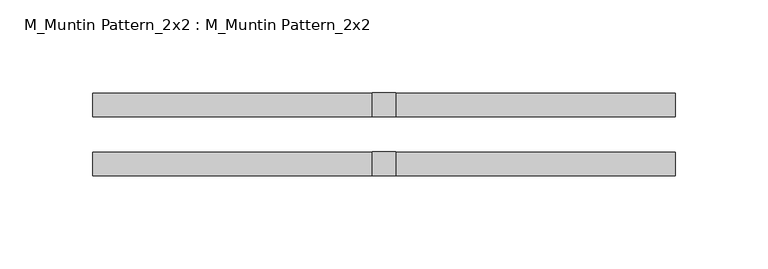
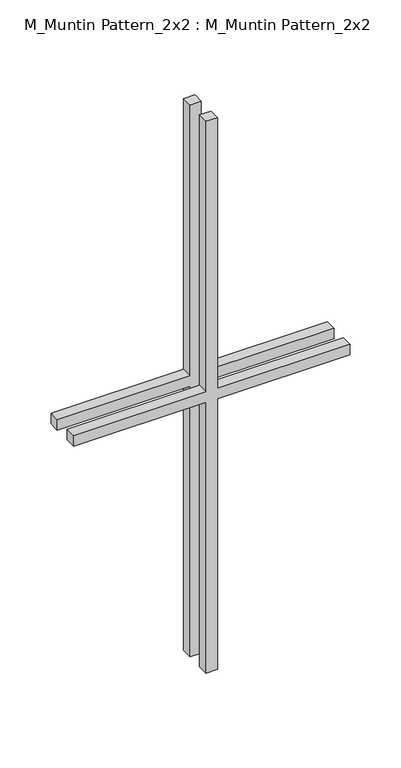
"""IFC4 building model written with IfcOpenShell, lengths in millimetres: proxy geometry, M_Muntin Pattern_2x2 : M_Muntin Pattern_2x2."""

from ifc_helpers import new_model, si_unit, frame, origin, place, context, project, spatial, polyline, outline, extrude, source, transform, mapped, element, save


def m_muntin_pattern_2x2_m_muntin_pattern_2x2_9259c5e2(model_context):
    return source(origin(), model_context, "Body", "SweptSolid", [
        extrude(outline(polyline([(336.5, -6.35), (336.5, -156.6333333), (323.8, -156.6333333), (323.8, -6.35), (0.0, -6.35), (0.0, 6.35), (323.8, 6.35), (323.8, 156.6333333), (336.5, 156.6333333), (336.5, 6.35), (660.3, 6.35), (660.3, -6.35), (336.5, -6.35)])), frame((0.0, -22.225, 0.0), z_axis=(0.0, 1.0, 0.0), x_axis=(0.0, 0.0, 1.0)), (0.0, 0.0, 1.0), 12.7),
        extrude(outline(polyline([(336.5, -6.35), (336.5, -156.6333333), (323.8, -156.6333333), (323.8, -6.35), (0.0, -6.35), (0.0, 6.35), (323.8, 6.35), (323.8, 156.6333333), (336.5, 156.6333333), (336.5, 6.35), (660.3, 6.35), (660.3, -6.35), (336.5, -6.35)])), frame((0.0, 9.525, 0.0), z_axis=(0.0, 1.0, 0.0), x_axis=(0.0, 0.0, 1.0)), (0.0, 0.0, 1.0), 12.7),
    ])


if __name__ == "__main__":
    model = new_model("IFC4")
    model_context = context("Model", 3, world=origin())
    ifc_project = project(units=[si_unit("LENGTHUNIT", "METRE", prefix="MILLI")], contexts=[model_context])
    site = spatial("IfcSite", under=ifc_project)
    building = spatial("IfcBuilding", under=site)
    placement = place(None, origin())
    m_muntin_pattern_2x2_m_muntin_pattern_2x2_shape = m_muntin_pattern_2x2_m_muntin_pattern_2x2_9259c5e2(model_context)
    element("IfcBuildingElementProxy", 1, Name="M_Muntin Pattern_2x2 : M_Muntin Pattern_2x2", ObjectType="M_Muntin Pattern_2x2 : M_Muntin Pattern_2x2", at=placement, inside=building, context=model_context, shape_type="MappedRepresentation", body=[
        mapped(m_muntin_pattern_2x2_m_muntin_pattern_2x2_shape, transform((0.0, 0.0, 0.0), x_axis=(1.0, 0.0, 0.0), y_axis=(0.0, 1.0, 0.0), z_axis=(0.0, 0.0, 1.0))),
    ])
    save(model, "model.ifc")

# Revit data of these elements
# Type "M_Muntin Pattern_2x2 : M_Muntin Pattern_2x2"
#   Width [instance default] = 3' - 11.24409"
#   Thickness = 0' - 0 1/2"
#   Height [instance default] = 3' - 11.24409"
#   Distance = 0' - 0 3/4"
#   Interior Material [instance default] = none
#   Exterior Material [instance default] = none
#   Default Elevation = 0
# Element 1 (IfcBuildingElementProxy, "M_Muntin Pattern_2x2 : M_Muntin Pattern_2x2")
#   Width = 1' - 0.33333"
#   Height = 2' - 1.99606"
#   Interior Material = Wood - Stained
#   Exterior Material = Clad - White
#   Materials on its faces: "Clad - White", "Wood - Stained"
# Materials
#   "Clad - White": class "Wood", colour RGB 242 242 238, transparency 0, Cost = 0
#   "Wood - Stained": class "Wood", colour RGB 227 170 128, transparency 0, Cost = 0
